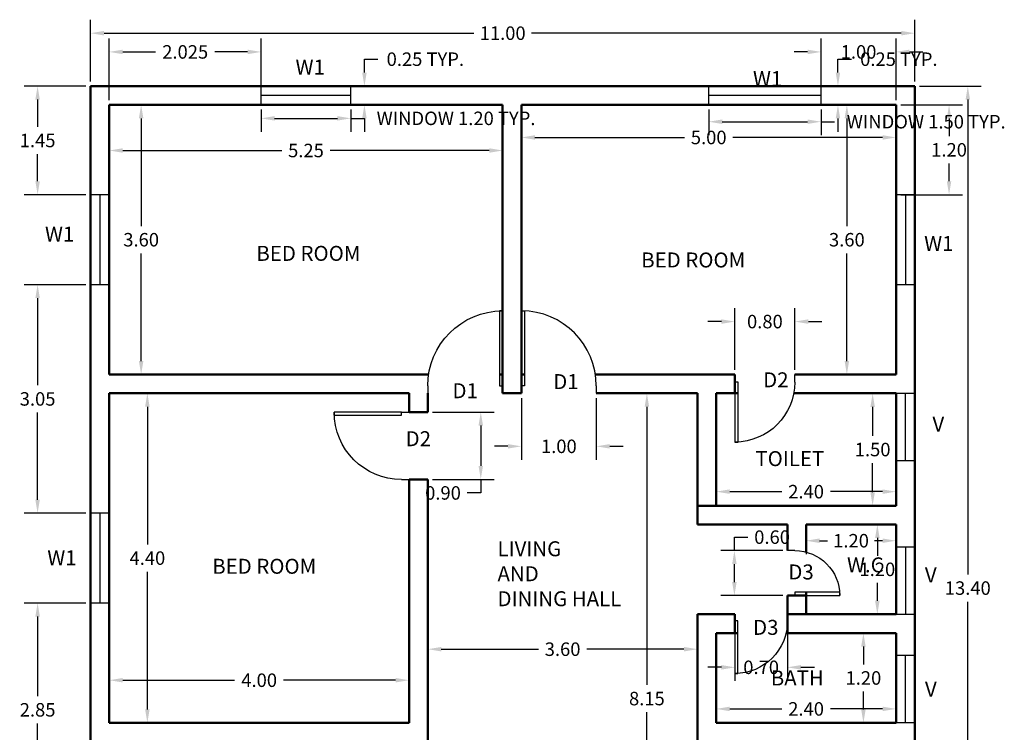
# Model space of a CAD drawing. Units: metres. Extents: x 136 to 273, y 211 to 430.
# Tile 2 of 2: x 136.09 to 149.23, y 216.67 to 226.18. Entities that reach past the tile are written whole.
import ezdxf

# ---------------------------------------------------------------- set-up
doc = ezdxf.new("R2010")
doc.units = ezdxf.units.M
doc.header["$MEASUREMENT"] = 0
for name, color, linetype, lineweight in [('A-ANNO-DIMS', 7, 'Continuous', 18), ('A-ANNO-TEXT', 221, 'Continuous', 18), ('A-AREA-IDEN', 221, 'Continuous', 25), ('DOOR', 240, 'Continuous', 25), ('VN', 172, 'Continuous', 25), ('WALL', 6, 'Continuous', 50), ('WD', 80, 'Continuous', 25)]:
    doc.layers.add(name, color=color, linetype=linetype, lineweight=lineweight)
doc.styles.get("Standard").update_dxf_attribs({"font": 'arial.ttf'})
doc.dimstyles.get("Standard").update_dxf_attribs({"dimtxt": 0.18, "dimasz": 0.18, "dimexe": 0.18, "dimexo": 0.0625, "dimgap": 0.09, "dimtad": 0, "dimtih": 1, "dimtoh": 1, "dimzin": 0, "dimdsep": 46, "dimtxsty": 'Standard', "dimcen": 0.09, "dimadec": 0, "dimazin": 0, "dimtfac": 1, "dimtofl": 0, "dimtmove": 0, "dimatfit": 3, "dimfxl": 1, "dimtolj": 1, "dimtzin": 0, "dimarcsym": 0})

# ---------------------------------------------------------------- blocks, each defined once
blk = doc.blocks.new('*U3')
for p, q in [((0, 0), (0, -100)), ((1000, 0), (1000, -100))]:
    blk.add_line(p, q)
blk.add_lwpolyline([(0, 0), (0, 1000), (43.75, 1000), (43.75, 0)], close=True)
blk.add_arc((0, 0), 1000, 0, 90)
blk = doc.blocks.new('*U4')
for p, q in [((0, 0), (0, -100)), ((900, 0), (900, -100))]:
    blk.add_line(p, q)
blk.add_lwpolyline([(0, 0), (0, 900), (43.75, 900), (43.75, 0)], close=True)
blk.add_arc((0, 0), 900, 0, 90)
blk = doc.blocks.new('*U5')
for p, q in [((0, 0), (0, -100)), ((800, 0), (800, -100))]:
    blk.add_line(p, q)
blk.add_lwpolyline([(0, 0), (0, 800), (43.75, 800), (43.75, 0)], close=True)
blk.add_arc((0, 0), 800, 0, 90)
blk = doc.blocks.new('*U6')
for p, q in [((0, 0), (0, -100)), ((600, 0), (600, -100))]:
    blk.add_line(p, q)
blk.add_lwpolyline([(0, 0), (0, 600), (43.75, 600), (43.75, 0)], close=True)
blk.add_arc((0, 0), 600, 0, 90)
blk = doc.blocks.new('*D7')
at = {"layer": 'A-ANNO-DIMS', "color": 0, "lineweight": -2, "transparency": 16777216}
for p, q in [((137.283, 224.984), (137.283, 224.258)), ((142.533, 224.984), (142.533, 224.258)), ((137.463, 224.438), (139.584, 224.438)), ((142.353, 224.438), (140.232, 224.438))]:
    blk.add_line(p, q, dxfattribs=at)
at = {"layer": 'A-ANNO-DIMS', "color": 0, "transparency": 16777216}
for points in [[(137.463, 224.468), (137.463, 224.408), (137.283, 224.438)], [(142.353, 224.468), (142.353, 224.408), (142.533, 224.438)]]:
    blk.add_solid(points, dxfattribs=at)
at = {"layer": 'Defpoints', "color": 0, "transparency": 16777216}
for p in [(137.283, 225.047), (142.533, 225.047), (142.533, 224.438)]:
    blk.add_point(p, dxfattribs=at)
at = {"layer": 'A-ANNO-DIMS', "color": 0, "transparency": 16777216, "insert": (139.908, 224.438), "char_height": 0.18, "attachment_point": 5}
blk.add_mtext('\\A1;5.25', dxfattribs=at)
blk = doc.blocks.new('*D8')
at = {"layer": 'A-ANNO-DIMS', "color": 0, "lineweight": -2, "transparency": 16777216}
for p, q in [((137.346, 225.047), (137.888, 225.047)), ((137.708, 224.867), (137.708, 223.429)), ((137.708, 221.627), (137.708, 223.065)), ((137.346, 221.447), (137.888, 221.447))]:
    blk.add_line(p, q, dxfattribs=at)
at = {"layer": 'A-ANNO-DIMS', "color": 0, "transparency": 16777216}
for points in [[(137.678, 224.867), (137.738, 224.867), (137.708, 225.047)], [(137.678, 221.627), (137.738, 221.627), (137.708, 221.447)]]:
    blk.add_solid(points, dxfattribs=at)
at = {"layer": 'Defpoints', "color": 0, "transparency": 16777216}
for p in [(137.283, 225.047), (137.283, 221.447), (137.708, 221.447)]:
    blk.add_point(p, dxfattribs=at)
at = {"layer": 'A-ANNO-DIMS', "color": 0, "transparency": 16777216, "insert": (137.708, 223.247), "char_height": 0.18, "attachment_point": 5}
blk.add_mtext('\\A1;3.60', dxfattribs=at)
blk = doc.blocks.new('*D9')
at = {"layer": 'A-ANNO-DIMS', "color": 0, "lineweight": -2, "transparency": 16777216}
for p, q in [((142.783, 224.984), (142.783, 224.432)), ((147.783, 224.984), (147.783, 224.432)), ((142.963, 224.612), (144.96, 224.612)), ((147.603, 224.612), (145.606, 224.612))]:
    blk.add_line(p, q, dxfattribs=at)
at = {"layer": 'A-ANNO-DIMS', "color": 0, "transparency": 16777216}
for points in [[(142.963, 224.642), (142.963, 224.582), (142.783, 224.612)], [(147.603, 224.642), (147.603, 224.582), (147.783, 224.612)]]:
    blk.add_solid(points, dxfattribs=at)
at = {"layer": 'Defpoints', "color": 0, "transparency": 16777216}
for p in [(142.783, 225.047), (147.783, 225.047), (147.783, 224.612)]:
    blk.add_point(p, dxfattribs=at)
at = {"layer": 'A-ANNO-DIMS', "color": 0, "transparency": 16777216, "insert": (145.283, 224.612), "char_height": 0.18, "attachment_point": 5}
blk.add_mtext('\\A1;5.00', dxfattribs=at)
blk = doc.blocks.new('*D10')
at = {"layer": 'A-ANNO-DIMS', "color": 0, "lineweight": -2, "transparency": 16777216}
for p, q in [((147.721, 225.047), (146.947, 225.047)), ((147.127, 224.867), (147.127, 223.429)), ((147.127, 221.627), (147.127, 223.065)), ((147.721, 221.447), (146.947, 221.447))]:
    blk.add_line(p, q, dxfattribs=at)
at = {"layer": 'A-ANNO-DIMS', "color": 0, "transparency": 16777216}
for points in [[(147.097, 224.867), (147.157, 224.867), (147.127, 225.047)], [(147.097, 221.627), (147.157, 221.627), (147.127, 221.447)]]:
    blk.add_solid(points, dxfattribs=at)
at = {"layer": 'Defpoints', "color": 0, "transparency": 16777216}
for p in [(147.127, 225.047), (147.783, 225.047), (147.783, 221.447)]:
    blk.add_point(p, dxfattribs=at)
at = {"layer": 'A-ANNO-DIMS', "color": 0, "transparency": 16777216, "insert": (147.127, 223.247), "char_height": 0.18, "attachment_point": 5}
blk.add_mtext('\\A1;3.60', dxfattribs=at)
blk = doc.blocks.new('*D11')
at = {"layer": 'A-ANNO-DIMS', "color": 0, "lineweight": -2, "transparency": 16777216}
for p, q in [((137.346, 221.197), (137.971, 221.197)), ((137.791, 221.017), (137.791, 219.179)), ((137.791, 216.977), (137.791, 218.815)), ((137.346, 216.797), (137.971, 216.797))]:
    blk.add_line(p, q, dxfattribs=at)
at = {"layer": 'A-ANNO-DIMS', "color": 0, "transparency": 16777216}
for points in [[(137.761, 221.017), (137.821, 221.017), (137.791, 221.197)], [(137.761, 216.977), (137.821, 216.977), (137.791, 216.797)]]:
    blk.add_solid(points, dxfattribs=at)
at = {"layer": 'Defpoints', "color": 0, "transparency": 16777216}
for p in [(137.283, 221.197), (137.791, 221.197), (137.283, 216.797)]:
    blk.add_point(p, dxfattribs=at)
at = {"layer": 'A-ANNO-DIMS', "color": 0, "transparency": 16777216, "insert": (137.791, 218.997), "char_height": 0.18, "attachment_point": 5}
blk.add_mtext('\\A1;4.40', dxfattribs=at)
blk = doc.blocks.new('*D12')
at = {"layer": 'A-ANNO-DIMS', "color": 0, "lineweight": -2, "transparency": 16777216}
for p, q in [((137.283, 216.859), (137.283, 217.547)), ((141.283, 216.859), (141.283, 217.547)), ((137.463, 217.367), (138.956, 217.367)), ((141.103, 217.367), (139.61, 217.367))]:
    blk.add_line(p, q, dxfattribs=at)
at = {"layer": 'A-ANNO-DIMS', "color": 0, "transparency": 16777216}
for points in [[(137.463, 217.397), (137.463, 217.337), (137.283, 217.367)], [(141.103, 217.397), (141.103, 217.337), (141.283, 217.367)]]:
    blk.add_solid(points, dxfattribs=at)
at = {"layer": 'Defpoints', "color": 0, "transparency": 16777216}
for p in [(137.283, 217.367), (137.283, 216.797), (141.283, 216.797)]:
    blk.add_point(p, dxfattribs=at)
at = {"layer": 'A-ANNO-DIMS', "color": 0, "transparency": 16777216, "insert": (139.283, 217.367), "char_height": 0.18, "attachment_point": 5}
blk.add_mtext('\\A1;4.00', dxfattribs=at)
blk = doc.blocks.new('*D17')
at = {"layer": 'A-ANNO-DIMS', "color": 0, "lineweight": -2, "transparency": 16777216}
for p, q in [((145.383, 216.859), (145.383, 217.164)), ((147.783, 216.859), (147.783, 217.164)), ((145.563, 216.984), (146.258, 216.984)), ((147.603, 216.984), (146.908, 216.984))]:
    blk.add_line(p, q, dxfattribs=at)
at = {"layer": 'A-ANNO-DIMS', "color": 0, "transparency": 16777216}
for points in [[(145.563, 217.014), (145.563, 216.954), (145.383, 216.984)], [(147.603, 217.014), (147.603, 216.954), (147.783, 216.984)]]:
    blk.add_solid(points, dxfattribs=at)
at = {"layer": 'Defpoints', "color": 0, "transparency": 16777216}
for p in [(145.383, 216.984), (145.383, 216.797), (147.783, 216.797)]:
    blk.add_point(p, dxfattribs=at)
at = {"layer": 'A-ANNO-DIMS', "color": 0, "transparency": 16777216, "insert": (146.583, 216.984), "char_height": 0.18, "attachment_point": 5}
blk.add_mtext('\\A1;2.40', dxfattribs=at)
blk = doc.blocks.new('*D18')
at = {"layer": 'A-ANNO-DIMS', "color": 0, "lineweight": -2, "transparency": 16777216}
for p, q in [((147.721, 217.997), (147.168, 217.997)), ((147.348, 217.817), (147.348, 217.579)), ((147.348, 216.977), (147.348, 217.215)), ((147.721, 216.797), (147.168, 216.797))]:
    blk.add_line(p, q, dxfattribs=at)
at = {"layer": 'A-ANNO-DIMS', "color": 0, "transparency": 16777216}
for points in [[(147.318, 217.817), (147.378, 217.817), (147.348, 217.997)], [(147.318, 216.977), (147.378, 216.977), (147.348, 216.797)]]:
    blk.add_solid(points, dxfattribs=at)
at = {"layer": 'Defpoints', "color": 0, "transparency": 16777216}
for p in [(147.783, 217.997), (147.348, 216.797), (147.783, 216.797)]:
    blk.add_point(p, dxfattribs=at)
at = {"layer": 'A-ANNO-DIMS', "color": 0, "transparency": 16777216, "insert": (147.348, 217.397), "char_height": 0.18, "attachment_point": 5}
blk.add_mtext('\\A1;1.20', dxfattribs=at)
blk = doc.blocks.new('*D19')
at = {"layer": 'A-ANNO-DIMS', "color": 0, "lineweight": -2, "transparency": 16777216}
for p, q in [((147.721, 219.447), (147.354, 219.447)), ((147.534, 219.267), (147.534, 219.029)), ((147.534, 218.427), (147.534, 218.665)), ((147.721, 218.247), (147.354, 218.247))]:
    blk.add_line(p, q, dxfattribs=at)
at = {"layer": 'A-ANNO-DIMS', "color": 0, "transparency": 16777216}
for points in [[(147.504, 219.267), (147.564, 219.267), (147.534, 219.447)], [(147.504, 218.427), (147.564, 218.427), (147.534, 218.247)]]:
    blk.add_solid(points, dxfattribs=at)
at = {"layer": 'Defpoints', "color": 0, "transparency": 16777216}
for p in [(147.534, 219.447), (147.783, 219.447), (147.783, 218.247)]:
    blk.add_point(p, dxfattribs=at)
at = {"layer": 'A-ANNO-DIMS', "color": 0, "transparency": 16777216, "insert": (147.534, 218.847), "char_height": 0.18, "attachment_point": 5}
blk.add_mtext('\\A1;1.20', dxfattribs=at)
blk = doc.blocks.new('*D20')
at = {"layer": 'A-ANNO-DIMS', "color": 0, "lineweight": -2, "transparency": 16777216}
for p, q in [((146.583, 219.384), (146.583, 219.049)), ((147.783, 219.384), (147.783, 219.049)), ((146.763, 219.229), (146.868, 219.229)), ((147.603, 219.229), (147.498, 219.229))]:
    blk.add_line(p, q, dxfattribs=at)
at = {"layer": 'A-ANNO-DIMS', "color": 0, "transparency": 16777216}
for points in [[(146.763, 219.259), (146.763, 219.199), (146.583, 219.229)], [(147.603, 219.259), (147.603, 219.199), (147.783, 219.229)]]:
    blk.add_solid(points, dxfattribs=at)
at = {"layer": 'Defpoints', "color": 0, "transparency": 16777216}
for p in [(146.583, 219.447), (147.783, 219.447), (147.783, 219.229)]:
    blk.add_point(p, dxfattribs=at)
at = {"layer": 'A-ANNO-DIMS', "color": 0, "transparency": 16777216, "insert": (147.183, 219.229), "char_height": 0.18, "attachment_point": 5}
blk.add_mtext('\\A1;1.20', dxfattribs=at)
blk = doc.blocks.new('*D21')
at = {"layer": 'A-ANNO-DIMS', "color": 0, "lineweight": -2, "transparency": 16777216}
for p, q in [((147.721, 221.195), (147.291, 221.195)), ((147.471, 221.015), (147.471, 220.628)), ((147.471, 219.877), (147.471, 220.264)), ((147.721, 219.697), (147.291, 219.697))]:
    blk.add_line(p, q, dxfattribs=at)
at = {"layer": 'A-ANNO-DIMS', "color": 0, "transparency": 16777216}
for points in [[(147.441, 221.015), (147.501, 221.015), (147.471, 221.195)], [(147.441, 219.877), (147.501, 219.877), (147.471, 219.697)]]:
    blk.add_solid(points, dxfattribs=at)
at = {"layer": 'Defpoints', "color": 0, "transparency": 16777216}
for p in [(147.471, 221.195), (147.783, 221.195), (147.783, 219.697)]:
    blk.add_point(p, dxfattribs=at)
at = {"layer": 'A-ANNO-DIMS', "color": 0, "transparency": 16777216, "insert": (147.471, 220.446), "char_height": 0.18, "attachment_point": 5}
blk.add_mtext('\\A1;1.50', dxfattribs=at)
blk = doc.blocks.new('*D22')
at = {"layer": 'A-ANNO-DIMS', "color": 0, "lineweight": -2, "transparency": 16777216}
for p, q in [((145.383, 219.759), (145.383, 220.064)), ((147.783, 219.759), (147.783, 220.064)), ((145.563, 219.884), (146.258, 219.884)), ((147.603, 219.884), (146.908, 219.884))]:
    blk.add_line(p, q, dxfattribs=at)
at = {"layer": 'A-ANNO-DIMS', "color": 0, "transparency": 16777216}
for points in [[(145.563, 219.914), (145.563, 219.854), (145.383, 219.884)], [(147.603, 219.914), (147.603, 219.854), (147.783, 219.884)]]:
    blk.add_solid(points, dxfattribs=at)
at = {"layer": 'Defpoints', "color": 0, "transparency": 16777216}
for p in [(147.783, 219.884), (145.383, 219.697), (147.783, 219.697)]:
    blk.add_point(p, dxfattribs=at)
at = {"layer": 'A-ANNO-DIMS', "color": 0, "transparency": 16777216, "insert": (146.583, 219.884), "char_height": 0.18, "attachment_point": 5}
blk.add_mtext('\\A1;2.40', dxfattribs=at)
blk = doc.blocks.new('*D23')
at = {"layer": 'A-ANNO-DIMS', "color": 0, "lineweight": -2, "transparency": 16777216}
for p, q in [((141.533, 218.234), (141.533, 217.601)), ((145.133, 218.184), (145.133, 217.601)), ((141.713, 217.781), (143.01, 217.781)), ((144.953, 217.781), (143.656, 217.781))]:
    blk.add_line(p, q, dxfattribs=at)
at = {"layer": 'A-ANNO-DIMS', "color": 0, "transparency": 16777216}
for points in [[(141.713, 217.811), (141.713, 217.751), (141.533, 217.781)], [(144.953, 217.811), (144.953, 217.751), (145.133, 217.781)]]:
    blk.add_solid(points, dxfattribs=at)
at = {"layer": 'Defpoints', "color": 0, "transparency": 16777216}
for p in [(141.533, 218.297), (145.133, 218.247), (145.133, 217.781)]:
    blk.add_point(p, dxfattribs=at)
at = {"layer": 'A-ANNO-DIMS', "color": 0, "transparency": 16777216, "insert": (143.333, 217.781), "char_height": 0.18, "attachment_point": 5}
blk.add_mtext('\\A1;3.60', dxfattribs=at)
blk = doc.blocks.new('*D24')
at = {"layer": 'A-ANNO-DIMS', "color": 0, "lineweight": -2, "transparency": 16777216}
for p, q in [((144.521, 221.197), (144.638, 221.197)), ((144.458, 221.017), (144.458, 217.304)), ((144.458, 213.227), (144.458, 216.94)), ((144.521, 213.047), (144.638, 213.047))]:
    blk.add_line(p, q, dxfattribs=at)
at = {"layer": 'A-ANNO-DIMS', "color": 0, "transparency": 16777216}
for points in [[(144.428, 221.017), (144.488, 221.017), (144.458, 221.197)], [(144.428, 213.227), (144.488, 213.227), (144.458, 213.047)]]:
    blk.add_solid(points, dxfattribs=at)
at = {"layer": 'Defpoints', "color": 0, "transparency": 16777216}
for p in [(144.458, 221.197), (144.458, 213.047), (144.458, 213.047)]:
    blk.add_point(p, dxfattribs=at)
at = {"layer": 'A-ANNO-DIMS', "color": 0, "transparency": 16777216, "insert": (144.458, 217.122), "char_height": 0.18, "attachment_point": 5}
blk.add_mtext('\\A1;8.15', dxfattribs=at)
blk = doc.blocks.new('WIN-1200')
for p, q in [((0, 0), (0, 0.25)), ((1.2, 0), (1.2, 0.25)), ((1.2, 0.125), (0, 0.125))]:
    blk.add_line(p, q)
blk = doc.blocks.new('WIN-1500')
for p, q in [((0, 0), (0, 0.25)), ((1.5, 0), (1.5, 0.25)), ((1.5, 0.125), (0, 0.125))]:
    blk.add_line(p, q)
blk = doc.blocks.new('VENT-900')
for p, q in [((0, 0.9), (0.25, 0.9)), ((0.125, 0.9), (0.125, 0)), ((0, 0), (0.25, 0))]:
    blk.add_line(p, q)
blk = doc.blocks.new('*D28')
at = {"layer": 'A-ANNO-DIMS', "color": 0, "lineweight": -2, "transparency": 16777216}
for p, q in [((139.308, 224.984), (139.308, 224.687)), ((140.508, 224.984), (140.508, 224.687)), ((139.488, 224.867), (140.328, 224.867)), ((140.508, 224.867), (140.688, 224.867))]:
    blk.add_line(p, q, dxfattribs=at)
at = {"layer": 'A-ANNO-DIMS', "color": 0, "transparency": 16777216}
for points in [[(139.488, 224.897), (139.488, 224.837), (139.308, 224.867)], [(140.328, 224.897), (140.328, 224.837), (140.508, 224.867)]]:
    blk.add_solid(points, dxfattribs=at)
at = {"layer": 'Defpoints', "color": 0, "transparency": 16777216}
for p in [(139.308, 225.047), (140.508, 225.047), (140.508, 224.867)]:
    blk.add_point(p, dxfattribs=at)
at = {"layer": 'A-ANNO-DIMS', "color": 0, "transparency": 16777216, "insert": (141.911, 224.867), "char_height": 0.18, "attachment_point": 5}
blk.add_mtext('\\A1;WINDOW 1.20 TYP.', dxfattribs=at)
blk = doc.blocks.new('*D29')
at = {"layer": 'A-ANNO-DIMS', "color": 0, "lineweight": -2, "transparency": 16777216}
for p, q in [((140.688, 225.477), (140.688, 225.657)), ((140.688, 225.657), (140.868, 225.657)), ((140.571, 225.297), (140.868, 225.297)), ((140.571, 225.047), (140.868, 225.047)), ((140.688, 224.867), (140.688, 224.687))]:
    blk.add_line(p, q, dxfattribs=at)
at = {"layer": 'A-ANNO-DIMS', "color": 0, "transparency": 16777216}
for points in [[(140.658, 225.477), (140.718, 225.477), (140.688, 225.297)], [(140.658, 224.867), (140.718, 224.867), (140.688, 225.047)]]:
    blk.add_solid(points, dxfattribs=at)
at = {"layer": 'Defpoints', "color": 0, "transparency": 16777216}
for p in [(140.508, 225.297), (140.688, 225.297), (140.508, 225.047)]:
    blk.add_point(p, dxfattribs=at)
at = {"layer": 'A-ANNO-DIMS', "color": 0, "transparency": 16777216, "insert": (141.501, 225.657), "char_height": 0.18, "attachment_point": 5}
blk.add_mtext('\\A1;0.25 TYP.', dxfattribs=at)
blk = doc.blocks.new('*D30')
at = {"layer": 'A-ANNO-DIMS', "color": 0, "lineweight": -2, "transparency": 16777216}
for p, q in [((145.283, 224.984), (145.283, 224.642)), ((146.783, 224.984), (146.783, 224.642)), ((145.463, 224.822), (146.603, 224.822)), ((146.783, 224.822), (146.963, 224.822))]:
    blk.add_line(p, q, dxfattribs=at)
at = {"layer": 'A-ANNO-DIMS', "color": 0, "transparency": 16777216}
for points in [[(145.463, 224.852), (145.463, 224.792), (145.283, 224.822)], [(146.603, 224.852), (146.603, 224.792), (146.783, 224.822)]]:
    blk.add_solid(points, dxfattribs=at)
at = {"layer": 'Defpoints', "color": 0, "transparency": 16777216}
for p in [(145.283, 225.047), (146.783, 225.047), (146.783, 224.822)]:
    blk.add_point(p, dxfattribs=at)
at = {"layer": 'A-ANNO-DIMS', "color": 0, "transparency": 16777216, "insert": (148.186, 224.822), "char_height": 0.18, "attachment_point": 5}
blk.add_mtext('\\A1;WINDOW 1.50 TYP.', dxfattribs=at)
blk = doc.blocks.new('*D31')
at = {"layer": 'A-ANNO-DIMS', "color": 0, "lineweight": -2, "transparency": 16777216}
for p, q in [((147.008, 225.477), (147.008, 225.657)), ((147.008, 225.657), (147.188, 225.657)), ((146.846, 225.297), (147.188, 225.297)), ((146.846, 225.047), (147.188, 225.047)), ((147.008, 224.867), (147.008, 224.687))]:
    blk.add_line(p, q, dxfattribs=at)
at = {"layer": 'A-ANNO-DIMS', "color": 0, "transparency": 16777216}
for points in [[(146.978, 225.477), (147.038, 225.477), (147.008, 225.297)], [(146.978, 224.867), (147.038, 224.867), (147.008, 225.047)]]:
    blk.add_solid(points, dxfattribs=at)
at = {"layer": 'Defpoints', "color": 0, "transparency": 16777216}
for p in [(146.783, 225.297), (147.008, 225.297), (146.783, 225.047)]:
    blk.add_point(p, dxfattribs=at)
at = {"layer": 'A-ANNO-DIMS', "color": 0, "transparency": 16777216, "insert": (147.821, 225.657), "char_height": 0.18, "attachment_point": 5}
blk.add_mtext('\\A1;0.25 TYP.', dxfattribs=at)
blk = doc.blocks.new('*D34')
at = {"layer": 'A-ANNO-DIMS', "color": 0, "lineweight": -2, "transparency": 16777216}
for p, q in [((137.033, 225.359), (137.033, 226.184)), ((148.033, 225.359), (148.033, 226.184)), ((137.213, 226.004), (142.148, 226.004)), ((147.853, 226.004), (142.918, 226.004))]:
    blk.add_line(p, q, dxfattribs=at)
at = {"layer": 'A-ANNO-DIMS', "color": 0, "transparency": 16777216}
for points in [[(137.213, 226.034), (137.213, 225.974), (137.033, 226.004)], [(147.853, 226.034), (147.853, 225.974), (148.033, 226.004)]]:
    blk.add_solid(points, dxfattribs=at)
at = {"layer": 'Defpoints', "color": 0, "transparency": 16777216}
for p in [(148.033, 226.004), (137.033, 225.297), (148.033, 225.297)]:
    blk.add_point(p, dxfattribs=at)
at = {"layer": 'A-ANNO-DIMS', "color": 0, "transparency": 16777216, "insert": (142.533, 226.004), "char_height": 0.18, "attachment_point": 5}
blk.add_mtext('\\A1;11.00', dxfattribs=at)
blk = doc.blocks.new('*D35')
at = {"layer": 'A-ANNO-DIMS', "color": 0, "lineweight": -2, "transparency": 16777216}
for p, q in [((148.096, 225.297), (148.921, 225.297)), ((148.741, 225.117), (148.741, 218.779)), ((148.741, 212.077), (148.741, 218.415)), ((143.146, 211.897), (148.921, 211.897))]:
    blk.add_line(p, q, dxfattribs=at)
at = {"layer": 'A-ANNO-DIMS', "color": 0, "transparency": 16777216}
for points in [[(148.711, 225.117), (148.771, 225.117), (148.741, 225.297)], [(148.711, 212.077), (148.771, 212.077), (148.741, 211.897)]]:
    blk.add_solid(points, dxfattribs=at)
at = {"layer": 'Defpoints', "color": 0, "transparency": 16777216}
for p in [(148.033, 225.297), (148.741, 225.297), (143.083, 211.897)]:
    blk.add_point(p, dxfattribs=at)
at = {"layer": 'A-ANNO-DIMS', "color": 0, "transparency": 16777216, "insert": (148.741, 218.597), "char_height": 0.18, "attachment_point": 5}
blk.add_mtext('\\A1;13.40', dxfattribs=at)
blk = doc.blocks.new('*D39')
at = {"layer": 'A-ANNO-DIMS', "color": 0, "lineweight": -2, "transparency": 16777216}
for p, q in [((137.283, 225.109), (137.283, 225.934)), ((139.308, 225.109), (139.308, 225.934)), ((137.463, 225.754), (137.9, 225.754)), ((139.128, 225.754), (138.691, 225.754))]:
    blk.add_line(p, q, dxfattribs=at)
at = {"layer": 'A-ANNO-DIMS', "color": 0, "transparency": 16777216}
for points in [[(137.463, 225.784), (137.463, 225.724), (137.283, 225.754)], [(139.128, 225.784), (139.128, 225.724), (139.308, 225.754)]]:
    blk.add_solid(points, dxfattribs=at)
at = {"layer": 'Defpoints', "color": 0, "transparency": 16777216}
for p in [(139.308, 225.754), (137.283, 225.047), (139.308, 225.047)]:
    blk.add_point(p, dxfattribs=at)
at = {"layer": 'A-ANNO-DIMS', "color": 0, "transparency": 16777216, "insert": (138.296, 225.754), "char_height": 0.18, "attachment_point": 5}
blk.add_mtext('\\A1;2.025', dxfattribs=at)
blk = doc.blocks.new('*D40')
at = {"layer": 'A-ANNO-DIMS', "color": 0, "lineweight": -2, "transparency": 16777216}
for p, q in [((146.783024, 225.109143), (146.783024, 225.934143)), ((147.783024, 225.109143), (147.783024, 225.934143)), ((146.603024, 225.754143), (146.423024, 225.754143)), ((147.963024, 225.754143), (148.143024, 225.754143))]:
    blk.add_line(p, q, dxfattribs=at)
at = {"layer": 'A-ANNO-DIMS', "color": 0, "transparency": 16777216}
for points in [[(146.603024, 225.784143), (146.603024, 225.724143), (146.783024, 225.754143)], [(147.963024, 225.784143), (147.963024, 225.724143), (147.783024, 225.754143)]]:
    blk.add_solid(points, dxfattribs=at)
at = {"layer": 'Defpoints', "color": 0, "transparency": 16777216}
for p in [(147.783024, 225.754143), (146.783024, 225.046643), (147.783024, 225.046643)]:
    blk.add_point(p, dxfattribs=at)
at = {"layer": 'A-ANNO-DIMS', "color": 0, "transparency": 16777216, "insert": (147.283024, 225.754143), "char_height": 0.18, "attachment_point": 5}
blk.add_mtext('\\A1;1.00', dxfattribs=at)
blk = doc.blocks.new('*D41')
at = {"layer": 'A-ANNO-DIMS', "color": 0, "lineweight": -2, "transparency": 16777216}
for p, q in [((136.971, 225.297), (136.146, 225.297)), ((136.326, 225.117), (136.326, 224.754)), ((136.326, 224.027), (136.326, 224.39)), ((136.971, 223.847), (136.146, 223.847))]:
    blk.add_line(p, q, dxfattribs=at)
at = {"layer": 'A-ANNO-DIMS', "color": 0, "transparency": 16777216}
for points in [[(136.296, 225.117), (136.356, 225.117), (136.326, 225.297)], [(136.296, 224.027), (136.356, 224.027), (136.326, 223.847)]]:
    blk.add_solid(points, dxfattribs=at)
at = {"layer": 'Defpoints', "color": 0, "transparency": 16777216}
for p in [(136.326, 225.297), (137.033, 225.297), (137.033, 223.847)]:
    blk.add_point(p, dxfattribs=at)
at = {"layer": 'A-ANNO-DIMS', "color": 0, "transparency": 16777216, "insert": (136.326, 224.572), "char_height": 0.18, "attachment_point": 5}
blk.add_mtext('\\A1;1.45', dxfattribs=at)
blk = doc.blocks.new('*D42')
at = {"layer": 'A-ANNO-DIMS', "color": 0, "lineweight": -2, "transparency": 16777216}
for p, q in [((136.971, 222.647), (136.146, 222.647)), ((136.326, 222.467), (136.326, 221.304)), ((136.326, 219.777), (136.326, 220.94)), ((136.971, 219.597), (136.146, 219.597))]:
    blk.add_line(p, q, dxfattribs=at)
at = {"layer": 'A-ANNO-DIMS', "color": 0, "transparency": 16777216}
for points in [[(136.296, 222.467), (136.356, 222.467), (136.326, 222.647)], [(136.296, 219.777), (136.356, 219.777), (136.326, 219.597)]]:
    blk.add_solid(points, dxfattribs=at)
at = {"layer": 'Defpoints', "color": 0, "transparency": 16777216}
for p in [(136.326, 222.647), (137.033, 222.647), (137.033, 219.597)]:
    blk.add_point(p, dxfattribs=at)
at = {"layer": 'A-ANNO-DIMS', "color": 0, "transparency": 16777216, "insert": (136.326, 221.122), "char_height": 0.18, "attachment_point": 5}
blk.add_mtext('\\A1;3.05', dxfattribs=at)
blk = doc.blocks.new('*D43')
at = {"layer": 'A-ANNO-DIMS', "color": 0, "lineweight": -2, "transparency": 16777216}
for p, q in [((136.971, 218.397), (136.146, 218.397)), ((136.326, 218.217), (136.326, 217.154)), ((136.326, 215.727), (136.326, 216.79)), ((136.971, 215.547), (136.146, 215.547))]:
    blk.add_line(p, q, dxfattribs=at)
at = {"layer": 'A-ANNO-DIMS', "color": 0, "transparency": 16777216}
for points in [[(136.296, 218.217), (136.356, 218.217), (136.326, 218.397)], [(136.296, 215.727), (136.356, 215.727), (136.326, 215.547)]]:
    blk.add_solid(points, dxfattribs=at)
at = {"layer": 'Defpoints', "color": 0, "transparency": 16777216}
for p in [(136.326, 218.397), (137.033, 218.397), (137.033, 215.547)]:
    blk.add_point(p, dxfattribs=at)
at = {"layer": 'A-ANNO-DIMS', "color": 0, "transparency": 16777216, "insert": (136.326, 216.972), "char_height": 0.18, "attachment_point": 5}
blk.add_mtext('\\A1;2.85', dxfattribs=at)
blk = doc.blocks.new('*D45')
at = {"layer": 'A-ANNO-DIMS', "color": 0, "lineweight": -2, "transparency": 16777216}
for p, q in [((147.846, 225.047), (148.671, 225.047)), ((148.491, 224.867), (148.491, 224.629)), ((148.491, 224.027), (148.491, 224.265)), ((147.846, 223.847), (148.671, 223.847))]:
    blk.add_line(p, q, dxfattribs=at)
at = {"layer": 'A-ANNO-DIMS', "color": 0, "transparency": 16777216}
for points in [[(148.461, 224.867), (148.521, 224.867), (148.491, 225.047)], [(148.461, 224.027), (148.521, 224.027), (148.491, 223.847)]]:
    blk.add_solid(points, dxfattribs=at)
at = {"layer": 'Defpoints', "color": 0, "transparency": 16777216}
for p in [(147.783, 225.047), (147.783, 223.847), (148.491, 223.847)]:
    blk.add_point(p, dxfattribs=at)
at = {"layer": 'A-ANNO-DIMS', "color": 0, "transparency": 16777216, "insert": (148.491, 224.447), "char_height": 0.18, "attachment_point": 5}
blk.add_mtext('\\A1;1.20', dxfattribs=at)
blk = doc.blocks.new('*D50')
at = {"layer": 'A-ANNO-DIMS', "color": 0, "lineweight": -2, "transparency": 16777216}
for p, q in [((142.783024, 221.134143), (142.783024, 220.309143)), ((143.783024, 221.134143), (143.783024, 220.309143)), ((142.603024, 220.489143), (142.423024, 220.489143)), ((143.963024, 220.489143), (144.143024, 220.489143))]:
    blk.add_line(p, q, dxfattribs=at)
at = {"layer": 'A-ANNO-DIMS', "color": 0, "transparency": 16777216}
for points in [[(142.603024, 220.519143), (142.603024, 220.459143), (142.783024, 220.489143)], [(143.963024, 220.519143), (143.963024, 220.459143), (143.783024, 220.489143)]]:
    blk.add_solid(points, dxfattribs=at)
at = {"layer": 'Defpoints', "color": 0, "transparency": 16777216}
for p in [(142.783024, 221.196643), (143.783024, 221.196643), (142.783024, 220.489143)]:
    blk.add_point(p, dxfattribs=at)
at = {"layer": 'A-ANNO-DIMS', "color": 0, "transparency": 16777216, "insert": (143.283024, 220.489143), "char_height": 0.18, "attachment_point": 5}
blk.add_mtext('\\A1;1.00', dxfattribs=at)
blk = doc.blocks.new('*D51')
at = {"layer": 'A-ANNO-DIMS', "color": 0, "lineweight": -2, "transparency": 16777216}
for p, q in [((141.596, 220.947), (142.421, 220.947)), ((142.241, 220.767), (142.241, 220.227)), ((141.596, 220.047), (142.421, 220.047)), ((142.241, 220.047), (142.241, 219.867)), ((142.241, 219.867), (142.061, 219.867))]:
    blk.add_line(p, q, dxfattribs=at)
at = {"layer": 'A-ANNO-DIMS', "color": 0, "transparency": 16777216}
for points in [[(142.211, 220.767), (142.271, 220.767), (142.241, 220.947)], [(142.211, 220.227), (142.271, 220.227), (142.241, 220.047)]]:
    blk.add_solid(points, dxfattribs=at)
at = {"layer": 'Defpoints', "color": 0, "transparency": 16777216}
for p in [(141.533, 220.947), (141.533, 220.047), (142.241, 220.047)]:
    blk.add_point(p, dxfattribs=at)
at = {"layer": 'A-ANNO-DIMS', "color": 0, "transparency": 16777216, "insert": (141.737, 219.867), "char_height": 0.18, "attachment_point": 5}
blk.add_mtext('\\A1;0.90', dxfattribs=at)
blk = doc.blocks.new('*D52')
at = {"layer": 'A-ANNO-DIMS', "color": 0, "lineweight": -2, "transparency": 16777216}
for p, q in [((145.633024, 221.509143), (145.633024, 222.334143)), ((146.433024, 221.509143), (146.433024, 222.334143)), ((145.453024, 222.154143), (145.273024, 222.154143)), ((146.613024, 222.154143), (146.793024, 222.154143))]:
    blk.add_line(p, q, dxfattribs=at)
at = {"layer": 'A-ANNO-DIMS', "color": 0, "transparency": 16777216}
for points in [[(145.453024, 222.184143), (145.453024, 222.124143), (145.633024, 222.154143)], [(146.613024, 222.184143), (146.613024, 222.124143), (146.433024, 222.154143)]]:
    blk.add_solid(points, dxfattribs=at)
at = {"layer": 'Defpoints', "color": 0, "transparency": 16777216}
for p in [(146.433024, 222.154143), (145.633024, 221.446643), (146.433024, 221.446643)]:
    blk.add_point(p, dxfattribs=at)
at = {"layer": 'A-ANNO-DIMS', "color": 0, "transparency": 16777216, "insert": (146.033024, 222.154143), "char_height": 0.18, "attachment_point": 5}
blk.add_mtext('\\A1;0.80', dxfattribs=at)
blk = doc.blocks.new('*D53')
at = {"layer": 'A-ANNO-DIMS', "color": 0, "lineweight": -2, "transparency": 16777216}
for p, q in [((145.633024, 218.184143), (145.633024, 217.359143)), ((146.333024, 218.184143), (146.333024, 217.359143)), ((145.453024, 217.539143), (145.273024, 217.539143)), ((146.513024, 217.539143), (146.693024, 217.539143))]:
    blk.add_line(p, q, dxfattribs=at)
at = {"layer": 'A-ANNO-DIMS', "color": 0, "transparency": 16777216}
for points in [[(145.453024, 217.569143), (145.453024, 217.509143), (145.633024, 217.539143)], [(146.513024, 217.569143), (146.513024, 217.509143), (146.333024, 217.539143)]]:
    blk.add_solid(points, dxfattribs=at)
at = {"layer": 'Defpoints', "color": 0, "transparency": 16777216}
for p in [(145.633024, 218.246643), (146.333024, 218.246643), (145.633024, 217.539143)]:
    blk.add_point(p, dxfattribs=at)
at = {"layer": 'A-ANNO-DIMS', "color": 0, "transparency": 16777216, "insert": (145.983024, 217.539143), "char_height": 0.18, "attachment_point": 5}
blk.add_mtext('\\A1;0.70', dxfattribs=at)
blk = doc.blocks.new('*D54')
at = {"layer": 'A-ANNO-DIMS', "color": 0, "lineweight": -2, "transparency": 16777216}
for p, q in [((145.626, 219.097), (145.626, 219.277)), ((145.626, 219.277), (145.806, 219.277)), ((146.271, 219.097), (145.446, 219.097)), ((145.626, 218.677), (145.626, 218.917)), ((146.271, 218.497), (145.446, 218.497))]:
    blk.add_line(p, q, dxfattribs=at)
at = {"layer": 'A-ANNO-DIMS', "color": 0, "transparency": 16777216}
for points in [[(145.596, 218.917), (145.656, 218.917), (145.626, 219.097)], [(145.596, 218.677), (145.656, 218.677), (145.626, 218.497)]]:
    blk.add_solid(points, dxfattribs=at)
at = {"layer": 'Defpoints', "color": 0, "transparency": 16777216}
for p in [(145.626, 219.097), (146.333, 219.097), (146.333, 218.497)]:
    blk.add_point(p, dxfattribs=at)
at = {"layer": 'A-ANNO-DIMS', "color": 0, "transparency": 16777216, "insert": (146.129, 219.277), "char_height": 0.18, "attachment_point": 5}
blk.add_mtext('\\A1;0.60', dxfattribs=at)

msp = doc.modelspace()

# ---------------------------------------------------------------- linework, layer by layer
at = {"layer": 'WALL'}
for p, q in [((137.033, 225.2966), (142.783, 225.2966)), ((137.033, 221.1966), (137.033, 225.2966)), ((142.783, 225.2966), (148.033, 225.2966)), ((148.033, 225.2966), (148.033, 221.1966)), ((137.283, 225.0466), (142.533, 225.0466)), ((137.283, 221.4466), (137.283, 225.0466)), ((142.533, 225.0466), (142.533, 221.1966)), ((142.783, 225.0466), (142.783, 221.1966)), ((142.783, 225.0466), (147.783, 225.0466)), ((147.783, 225.0466), (147.783, 221.4466)), ((141.5443, 221.4466), (137.283, 221.4466)), ((142.533, 221.4466), (142.4893, 221.4466)), ((142.783, 221.4466), (142.8268, 221.4466)), ((143.7717, 221.4466), (145.633, 221.4466)), ((145.633, 221.4466), (145.633, 221.1966)), ((146.433, 221.4466), (147.783, 221.4466)), ((137.033, 221.1966), (137.033, 216.5466)), ((137.283, 221.1966), (137.283, 216.7966)), ((141.283, 221.1966), (137.283, 221.1966)), ((141.283, 221.1966), (141.283, 220.9466)), ((141.533, 221.1966), (141.533, 220.9466)), ((142.783, 221.1966), (142.533, 221.1966)), ((143.783, 221.1966), (145.133, 221.1966)), ((145.133, 221.1966), (145.133, 219.4466)), ((145.383, 221.1966), (145.383, 219.6966)), ((145.383, 221.1966), (145.6768, 221.1966)), ((146.4188, 221.1966), (147.783, 221.1966)), ((147.783, 221.1966), (147.783, 219.6966)), ((148.033, 221.1966), (148.033, 219.4466)), ((141.533, 220.9466), (141.283, 220.9466)), ((141.533, 220.0466), (141.283, 220.0466)), ((141.283, 220.0466), (141.283, 216.7966)), ((141.533, 220.0466), (141.533, 216.5466)), ((145.133, 219.6966), (147.783, 219.6966)), ((145.133, 219.4466), (146.333, 219.4466)), ((146.333, 219.4466), (146.333, 219.0966)), ((146.583, 219.4466), (146.583, 219.0776)), ((146.583, 219.4466), (147.783, 219.4466)), ((147.783, 219.4466), (147.783, 218.2466)), ((148.033, 219.4466), (148.033, 217.9966)), ((146.333, 218.4966), (146.583, 218.4966)), ((146.333, 218.4966), (146.333, 217.9966)), ((146.583, 218.5404), (146.583, 218.2466)), ((145.133, 218.2466), (145.133, 216.5466)), ((145.133, 218.2466), (145.633, 218.2466)), ((145.633, 218.2466), (145.633, 217.9966)), ((146.333, 218.2466), (147.783, 218.2466)), ((146.333, 218.2466), (146.3349, 218.2466)), ((146.583, 218.2466), (147.783, 218.2466)), ((145.383, 217.9966), (145.6714, 217.9966)), ((145.383, 217.9966), (145.383, 216.7966)), ((146.3158, 217.9966), (147.783, 217.9966)), ((147.783, 217.9966), (147.783, 216.7966)), ((148.033, 217.9966), (148.033, 216.5466)), ((141.283, 216.7966), (137.283, 216.7966)), ((145.383, 216.7966), (147.783, 216.7966))]:
    msp.add_line(p, q, dxfattribs=at)

# ---------------------------------------------------------------- block references
at = {"layer": 'DOOR', "extrusion": (0, 0, -1), "yscale": 0.001, "zscale": -0.001}
for p, xscale in [((-142.533, 221.2966), 0.001), ((-142.783, 221.2966), -0.001)]:
    msp.add_blockref('*U3', p, dxfattribs=dict(at, xscale=xscale))
at = {"layer": 'DOOR'}
for name, p, xscale, yscale, zscale, rotation in [('*U5', (145.633, 221.3466), -0.001, 0.001, 0.001, 180), ('*U4', (141.183, 220.9466), -0.001, 0.001, 0.001, 90), ('*U6', (146.433, 218.4966), -0.001, 0.001, 0.001, 270), ('*U5', (145.633, 218.1589), -0.0008772935854787, 0.0008772935854787, 0.0008772935854787, 180)]:
    msp.add_blockref(name, p, dxfattribs=dict(at, xscale=xscale, yscale=yscale, zscale=zscale, rotation=rotation))
at = {"layer": 'VN', "rotation": 180}
for p in [(148.033, 221.1954), (148.033, 217.6966)]:
    msp.add_blockref('VENT-900', p, dxfattribs=at)
at = {"layer": 'VN'}
msp.add_blockref('VENT-900', (147.783, 218.2466), dxfattribs=at)
at = {"layer": 'WD'}
for name, p in [('WIN-1200', (139.308, 225.0466)), ('WIN-1500', (145.283, 225.0466))]:
    msp.add_blockref(name, p, dxfattribs=at)
for p, rotation in [((137.283, 222.6466), 90), ((148.033, 222.6466), 90), ((137.283, 218.3966), 89.9999999999989)]:
    msp.add_blockref('WIN-1200', p, dxfattribs=dict(at, rotation=rotation))

# ---------------------------------------------------------------- texts
at = {"layer": 'A-ANNO-TEXT', "char_height": 0.2, "attachment_point": 1}
for s, width, insert in [('W1 ', 0.406895, (139.7687, 225.65)), ('W1 ', 0.406895, (145.8739, 225.4975)), ('W1 ', 0.406895, (136.4246, 223.4214)), ('W1 ', 0.406895, (148.1589, 223.2969)), ('D1 ', 0.276534, (143.208, 221.4527)), ('D2  ', 0.276534, (146.0097, 221.4768)), ('D1   ', 0.276534, (141.8632, 221.3312)), ('V ', 0.604517, (148.2693, 220.8854)), ('D2  ', 0.276534, (141.2376, 220.6909)), ('W1 ', 0.406895, (136.4554, 219.1014)), ('D3  ', 0.276534, (146.3459, 218.9121)), ('V ', 0.604517, (148.1686, 218.8721)), ('D3  ', 0.276534, (145.8752, 218.1725)), ('V ', 0.604517, (148.1697, 217.3472))]:
    msp.add_mtext_dynamic_manual_height_columns(s, width=width, gutter_width=1, heights=[0], dxfattribs=dict(at, insert=insert))
at = {"layer": 'A-AREA-IDEN', "char_height": 0.2, "attachment_point": 1}
for s, width, insert in [('\\pxqc;BED ROOM', 2.320368, (138.7803, 223.1649)), ('\\pxqc;BED ROOM', 2.320368, (143.9164, 223.0765)), ('\\pxqc;TOILET', 1.165601, (145.7827, 220.4249)), ('LIVING \\PAND\\PDINING HALL', 2.074494, (142.4642, 219.2215)), ('\\pxqc;BED ROOM', 2.320368, (138.1907, 218.9877)), (' W.C', 0.433353, (147.129, 219.0066)), ('\\pxqc;BATH', 0.894569, (146.018, 217.4974))]:
    msp.add_mtext_dynamic_manual_height_columns(s, width=width, gutter_width=1, heights=[0], dxfattribs=dict(at, insert=insert))

# ---------------------------------------------------------------- dimensions: what is measured, and where the dimension line sits
at = {"layer": 'A-ANNO-DIMS'}
for base, p1, p2, override, picture, middle in [((148.033, 226.0041), (137.033, 225.2966), (148.033, 225.2966), {"dimdec": 2, "dimlfac": 1, "dimrnd": 0, "dimzin": 0, "dimdsep": 46, "dimlunit": 2}, '*D34', (142.533, 226.0041)), ((139.308, 225.7541), (137.283, 225.0466), (139.308, 225.0466), {"dimdec": 3, "dimlfac": 1, "dimrnd": 0, "dimzin": 0, "dimdsep": 46, "dimlunit": 2}, '*D39', (138.2955, 225.7541)), ((142.533, 224.4384), (137.283, 225.0466), (142.533, 225.0466), {"dimclrd": 0, "dimclre": 0, "dimclrt": 0}, '*D7', (139.908, 224.4384)), ((147.783, 224.6125), (142.783, 225.0466), (147.783, 225.0466), {"dimclrd": 0, "dimclre": 0, "dimclrt": 0}, '*D9', (145.283, 224.6125)), ((146.433, 222.1541), (145.633, 221.4466), (146.433, 221.4466), {"dimdec": 2, "dimlfac": 1, "dimrnd": 0, "dimzin": 0, "dimdsep": 46, "dimlunit": 2}, '*D52', (146.033, 222.1541)), ((147.783, 219.8835), (145.383, 219.6966), (147.783, 219.6966), {"dimclrd": 0, "dimclre": 0, "dimclrt": 0}, '*D22', (146.583, 219.8835)), ((147.783, 219.2287), (146.583, 219.4466), (147.783, 219.4466), {"dimclrd": 0, "dimclre": 0, "dimclrt": 0}, '*D20', (147.183, 219.2287)), ((145.133, 217.7806), (141.533, 218.2966), (145.133, 218.2466), {"dimclrd": 0, "dimclre": 0, "dimclrt": 0}, '*D23', (143.333, 217.7806)), ((137.283, 217.3665), (141.283, 216.7966), (137.283, 216.7966), {"dimclrd": 0, "dimclre": 0, "dimclrt": 0}, '*D12', (139.283, 217.3665)), ((145.383, 216.9838), (147.783, 216.7966), (145.383, 216.7966), {"dimclrd": 0, "dimclre": 0, "dimclrt": 0}, '*D17', (146.583, 216.9838))]:
    dim = msp.add_linear_dim(base=base, p1=p1, p2=p2, dimstyle='Standard', override=override, dxfattribs=at)
    dim.commit()
    dim.dimension.update_dxf_attribs({"geometry": picture, "text_midpoint": middle})
for base, p1, p2, picture, middle in [((140.688, 225.2966), (140.508, 225.0466), (140.508, 225.2966), '*D29', (141.501, 225.6566)), ((147.008, 225.2966), (146.783, 225.0466), (146.783, 225.2966), '*D31', (147.821, 225.6566))]:
    dim = msp.add_linear_dim(base=base, p1=p1, p2=p2, angle=90, text='<> TYP.', dimstyle='Standard', override={"dimdec": 2, "dimlfac": 1, "dimrnd": 0, "dimzin": 0, "dimdsep": 46, "dimlunit": 2}, dxfattribs=at)
    dim.commit()
    dim.dimension.update_dxf_attribs({"geometry": picture, "text_midpoint": middle})
for base, p1, p2, angle, override, picture, middle in [((147.783, 225.7541), (146.783, 225.0466), (147.783, 225.0466), 0, {"dimdec": 2, "dimlfac": 1, "dimrnd": 0, "dimzin": 0, "dimdsep": 46, "dimlunit": 2}, '*D40', (147.283, 225.7541)), ((136.3255, 225.2966), (137.033, 223.8466), (137.033, 225.2966), 90, {"dimdec": 2, "dimlfac": 1, "dimrnd": 0, "dimzin": 0, "dimdsep": 46, "dimlunit": 2}, '*D41', (136.3255, 224.5716)), ((148.7405, 225.2966), (143.083, 211.8966), (148.033, 225.2966), 90, {"dimdec": 2, "dimlfac": 1, "dimrnd": 0, "dimzin": 0, "dimdsep": 46, "dimlunit": 2}, '*D35', (148.7405, 218.5966)), ((137.7077, 221.4466), (137.283, 225.0466), (137.283, 221.4466), 90, {"dimclrd": 0, "dimclre": 0, "dimclrt": 0}, '*D8', (137.7077, 223.2466)), ((147.1273, 225.0466), (147.783, 221.4466), (147.783, 225.0466), 90, {"dimclrd": 0, "dimclre": 0, "dimclrt": 0}, '*D10', (147.1273, 223.2466)), ((148.4905, 223.8466), (147.783, 225.0466), (147.783, 223.8466), 270, {"dimdec": 2, "dimlfac": 1, "dimrnd": 0, "dimzin": 0, "dimdsep": 46, "dimlunit": 2}, '*D45', (148.4905, 224.4466)), ((136.3255, 222.6466), (137.033, 219.5966), (137.033, 222.6466), 90, {"dimdec": 2, "dimlfac": 1, "dimrnd": 0, "dimzin": 0, "dimdsep": 46, "dimlunit": 2}, '*D42', (136.3255, 221.1216)), ((137.7909, 221.1966), (137.283, 216.7966), (137.283, 221.1966), 90, {"dimclrd": 0, "dimclre": 0, "dimclrt": 0}, '*D11', (137.7909, 218.9966)), ((142.783, 220.4891), (143.783, 221.1966), (142.783, 221.1966), 180, {"dimdec": 2, "dimlfac": 1, "dimrnd": 0, "dimzin": 0, "dimdsep": 46, "dimlunit": 2}, '*D50', (143.283, 220.4891)), ((144.458, 213.0466), (144.458, 221.1966), (144.458, 213.0466), 90, {"dimclrd": 0, "dimclre": 0, "dimclrt": 0}, '*D24', (144.458, 217.1216)), ((147.4708, 221.1954), (147.783, 219.6966), (147.783, 221.1954), 90, {"dimclrd": 0, "dimclre": 0, "dimclrt": 0}, '*D21', (147.4708, 220.446)), ((142.2405, 220.0466), (141.533, 220.9466), (141.533, 220.0466), 270, {"dimdec": 2, "dimlfac": 1, "dimrnd": 0, "dimzin": 0, "dimdsep": 46, "dimlunit": 2}, '*D51', (141.7371, 219.8666)), ((145.6255, 219.0966), (146.333, 218.4966), (146.333, 219.0966), 90, {"dimdec": 2, "dimlfac": 1, "dimrnd": 0, "dimzin": 0, "dimdsep": 46, "dimlunit": 2}, '*D54', (146.129, 219.2766)), ((147.5343, 219.4466), (147.783, 218.2466), (147.783, 219.4466), 90, {"dimclrd": 0, "dimclre": 0, "dimclrt": 0}, '*D19', (147.5343, 218.8466)), ((136.3255, 218.3966), (137.033, 215.5466), (137.033, 218.3966), 90, {"dimdec": 2, "dimlfac": 1, "dimrnd": 0, "dimzin": 0, "dimdsep": 46, "dimlunit": 2}, '*D43', (136.3255, 216.9716)), ((145.633, 217.5391), (146.333, 218.2466), (145.633, 218.2466), 180, {"dimdec": 2, "dimlfac": 1, "dimrnd": 0, "dimzin": 0, "dimdsep": 46, "dimlunit": 2}, '*D53', (145.983, 217.5391)), ((147.348, 216.7966), (147.783, 217.9966), (147.783, 216.7966), 90, {"dimclrd": 0, "dimclre": 0, "dimclrt": 0}, '*D18', (147.348, 217.3966))]:
    dim = msp.add_linear_dim(base=base, p1=p1, p2=p2, angle=angle, dimstyle='Standard', override=override, dxfattribs=at)
    dim.commit()
    dim.dimension.update_dxf_attribs({"geometry": picture, "text_midpoint": middle})
for base, p1, p2, picture, middle in [((140.508, 224.8666), (139.308, 225.0466), (140.508, 225.0466), '*D28', (141.9113, 224.8666)), ((146.783, 224.8216), (145.283, 225.0466), (146.783, 225.0466), '*D30', (148.1863, 224.8216))]:
    dim = msp.add_linear_dim(base=base, p1=p1, p2=p2, text='WINDOW <> TYP.', dimstyle='Standard', override={"dimdec": 2, "dimlfac": 1, "dimrnd": 0, "dimzin": 0, "dimdsep": 46, "dimlunit": 2}, dxfattribs=at)
    dim.commit()
    dim.dimension.update_dxf_attribs({"geometry": picture, "text_midpoint": middle})

doc.saveas('drawing.dxf')
